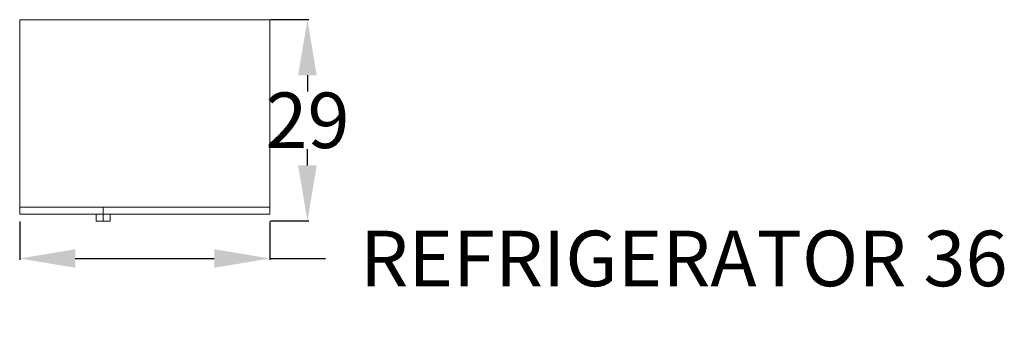
# Model space of a CAD drawing. Units: inches. Extents: x -52 to 678, y 23 to 685.
# Tile 9 of 11: x 186 to 328, y 639 to 685. Entities that reach past the tile are written whole.
import ezdxf

# ---------------------------------------------------------------- set-up
doc = ezdxf.new("R2010")
doc.units = ezdxf.units.IN
doc.header["$MEASUREMENT"] = 0
doc.layers.add('A-ANNO-DIMS', color=2, linetype='Continuous', lineweight=18)
doc.layers.add('A-EQPM', color=8, linetype='Continuous', lineweight=18)
doc.styles.get("Standard").update_dxf_attribs({"font": 'arial.ttf'})
doc.dimstyles.get("Standard").update_dxf_attribs({"dimtxt": 8, "dimasz": 8, "dimexe": 0.18, "dimexo": 0.0625, "dimgap": 0.09, "dimtad": 0, "dimtih": 1, "dimtoh": 1, "dimdec": 0, "dimzin": 0, "dimdsep": 46, "dimlunit": 3, "dimtxsty": 'Standard', "dimcen": 0.09, "dimadec": 0, "dimazin": 0, "dimtfac": 1, "dimtdec": 0, "dimtofl": 0, "dimtmove": 0, "dimatfit": 3, "dimfxl": 1, "dimtolj": 1, "dimtzin": 0, "dimarcsym": 0})

# ---------------------------------------------------------------- blocks, each defined once
blk = doc.blocks.new('Refrigerator-2 door - 36 in top')
for p, q in [((0, -26.999999), (36, -26.999999)), ((11, -27.999999), (11, -28.999999)), ((12, -26.999999), (12, -28.999999)), ((13, -28.999999), (13, -27.999999)), ((11, -28.999999), (13, -28.999999))]:
    blk.add_line(p, q)
blk.add_lwpolyline([(0, -27.999999), (0, 0), (36, 0), (36, -27.999999)], close=True)
blk = doc.blocks.new('*D27')
at = {"layer": 'A-ANNO-DIMS', "color": 0, "lineweight": -2, "transparency": 16777216}
for p, q in [((186.31, 656.18), (186.31, 650.67)), ((222.31, 656.18), (222.31, 650.67)), ((194.31, 650.85), (214.31, 650.85)), ((222.31, 650.85), (230.31, 650.85))]:
    blk.add_line(p, q, dxfattribs=at)
at = {"layer": 'A-ANNO-DIMS', "color": 0, "transparency": 16777216}
for points in [[(194.31, 652.18), (194.31, 649.51), (186.31, 650.85)], [(214.31, 652.18), (214.31, 649.51), (222.31, 650.85)]]:
    blk.add_solid(points, dxfattribs=at)
at = {"layer": 'Defpoints', "color": 0, "transparency": 16777216}
for p in [(186.31, 656.25), (222.31, 656.25), (222.31, 650.85)]:
    blk.add_point(p, dxfattribs=at)
at = {"layer": 'A-ANNO-DIMS', "color": 0, "transparency": 16777216, "insert": (281.87, 650.85), "char_height": 8, "attachment_point": 5}
blk.add_mtext('\\A1;REFRIGERATOR 36', dxfattribs=at)
blk = doc.blocks.new('*D28')
at = {"layer": 'A-ANNO-DIMS', "color": 0, "lineweight": -2, "transparency": 16777216}
for p, q in [((222.37, 685.25), (227.89, 685.25)), ((227.71, 677.25), (227.71, 674.92)), ((227.71, 664.25), (227.71, 666.57)), ((222.37, 656.25), (227.89, 656.25))]:
    blk.add_line(p, q, dxfattribs=at)
at = {"layer": 'A-ANNO-DIMS', "color": 0, "transparency": 16777216}
for points in [[(226.37, 677.25), (229.04, 677.25), (227.71, 685.25)], [(226.37, 664.25), (229.04, 664.25), (227.71, 656.25)]]:
    blk.add_solid(points, dxfattribs=at)
at = {"layer": 'Defpoints', "color": 0, "transparency": 16777216}
for p in [(222.31, 685.25), (227.71, 685.25), (222.31, 656.25)]:
    blk.add_point(p, dxfattribs=at)
at = {"layer": 'A-ANNO-DIMS', "color": 0, "transparency": 16777216, "insert": (227.71, 670.75), "char_height": 8, "attachment_point": 5}
blk.add_mtext('\\A1;29', dxfattribs=at)

msp = doc.modelspace()

# ---------------------------------------------------------------- block references
at = {"layer": 'A-EQPM'}
msp.add_blockref('Refrigerator-2 door - 36 in top', (186.3077, 685.2456), dxfattribs=at)

# ---------------------------------------------------------------- dimensions: what is measured, and where the dimension line sits
at = {"layer": 'A-ANNO-DIMS'}
dim = msp.add_linear_dim(base=(227.7077, 685.2456), p1=(222.3077, 656.2456), p2=(222.3077, 685.2456), angle=90, dimstyle='Standard', override={"dimdec": 0, "dimlfac": 1, "dimrnd": 0, "dimzin": 0, "dimdsep": 46, "dimlunit": 2}, dxfattribs=at)
dim.commit()
dim.dimension.update_dxf_attribs({"geometry": '*D28', "text_midpoint": (227.7077, 670.7456)})
dim = msp.add_linear_dim(base=(222.3077, 650.8456), p1=(186.3077, 656.2456), p2=(222.3077, 656.2456), text='REFRIGERATOR <>', dimstyle='Standard', override={"dimdec": 0, "dimlfac": 1, "dimrnd": 0, "dimzin": 0, "dimdsep": 46, "dimlunit": 2}, dxfattribs=at)
dim.commit()
dim.dimension.update_dxf_attribs({"geometry": '*D27', "text_midpoint": (281.8657, 650.8456)})

doc.saveas('drawing.dxf')
